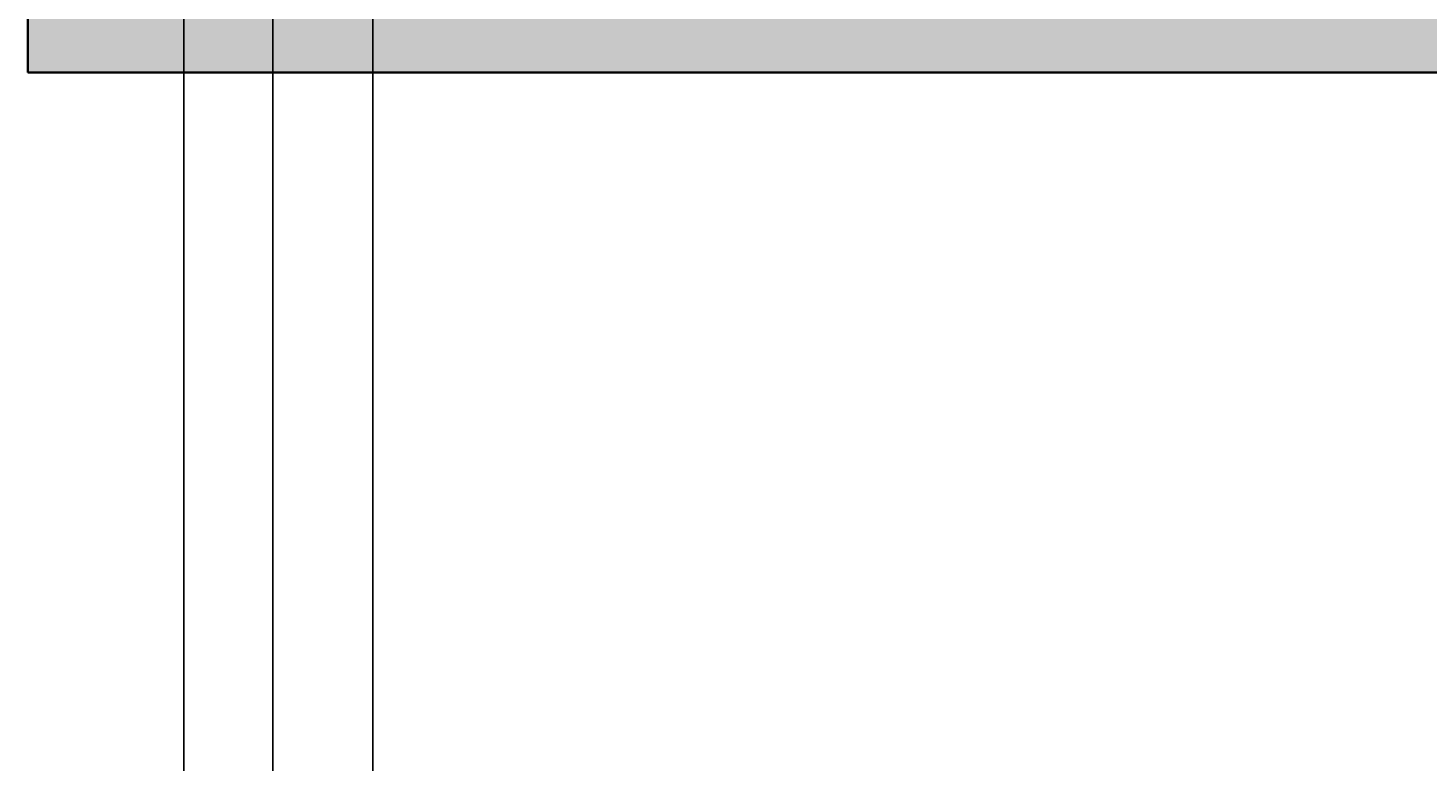
# Model space of a CAD drawing. Units: inches. Extents: x 1567 to 1964, y 1813 to 2447.
# Tile 22 of 28: x 1788 to 1851, y 2228 to 2261. Entities that reach past the tile are written whole.
import ezdxf

# ---------------------------------------------------------------- set-up
doc = ezdxf.new("R2010")
doc.units = ezdxf.units.IN
doc.layers.add('A-ANNO-DIMS', color=2, linetype='Continuous', lineweight=18)
doc.layers.add('A-WALL', color=7, linetype='Continuous', lineweight=35)
doc.layers.add('A-WALL-PATT', color=251, linetype='Continuous', lineweight=13, true_color=0x636466)
doc.styles.get("Standard").update_dxf_attribs({"font": 'arial.ttf'})
doc.dimstyles.get("Standard").update_dxf_attribs({"dimtxt": 0.18, "dimasz": 0.18, "dimexe": 0.18, "dimexo": 0.0625, "dimgap": 0.09, "dimtad": 0, "dimtih": 1, "dimtoh": 1, "dimdec": 4, "dimzin": 0, "dimdsep": 46, "dimtxsty": 'Standard', "dimcen": 0.09, "dimadec": 0, "dimazin": 0, "dimtfac": 1, "dimtdec": 4, "dimtofl": 0, "dimtmove": 0, "dimatfit": 3, "dimfxl": 1, "dimtolj": 1, "dimtzin": 0, "dimarcsym": 0})

# ---------------------------------------------------------------- blocks, each defined once
blk = doc.blocks.new('*D54')
at = {"layer": 'A-ANNO-DIMS', "color": 0, "lineweight": -2, "transparency": 16777216}
for p, q in [((1711.43, 1964.352), (1711.43, 2447.12)), ((1711.61, 2446.94), (1753.211, 2446.94)), ((1795.25, 2446.94), (1753.648, 2446.94)), ((1795.43, 1964.352), (1795.43, 2447.12))]:
    blk.add_line(p, q, dxfattribs=at)
at = {"layer": 'A-ANNO-DIMS', "color": 0, "transparency": 16777216}
for points in [[(1711.61, 2446.97), (1711.61, 2446.91), (1711.43, 2446.94)], [(1795.25, 2446.97), (1795.25, 2446.91), (1795.43, 2446.94)]]:
    blk.add_solid(points, dxfattribs=at)
at = {"layer": 'Defpoints', "color": 0, "transparency": 16777216}
for p in [(1795.43, 2446.94), (1711.43, 1964.29), (1795.43, 1964.29)]:
    blk.add_point(p, dxfattribs=at)
at = {"layer": 'A-ANNO-DIMS', "color": 0, "transparency": 16777216, "insert": (1753.43, 2446.94), "char_height": 0.18, "attachment_point": 5}
blk.add_mtext('\\A1;84', dxfattribs=at)
blk = doc.blocks.new('*D55')
at = {"layer": 'A-ANNO-DIMS', "color": 0, "lineweight": -2, "transparency": 16777216}
for p, q in [((1795.43, 1964.352), (1795.43, 2447.12)), ((1795.61, 2446.94), (1797.277, 2446.94)), ((1799.25, 2446.94), (1797.582, 2446.94)), ((1799.43, 1967.352), (1799.43, 2447.12))]:
    blk.add_line(p, q, dxfattribs=at)
at = {"layer": 'A-ANNO-DIMS', "color": 0, "transparency": 16777216}
for points in [[(1795.61, 2446.97), (1795.61, 2446.91), (1795.43, 2446.94)], [(1799.25, 2446.97), (1799.25, 2446.91), (1799.43, 2446.94)]]:
    blk.add_solid(points, dxfattribs=at)
at = {"layer": 'Defpoints', "color": 0, "transparency": 16777216}
for p in [(1799.43, 2446.94), (1799.43, 1967.29), (1795.43, 1964.29)]:
    blk.add_point(p, dxfattribs=at)
at = {"layer": 'A-ANNO-DIMS', "color": 0, "transparency": 16777216, "insert": (1797.43, 2446.94), "char_height": 0.18, "attachment_point": 5}
blk.add_mtext('\\A1;4', dxfattribs=at)
blk = doc.blocks.new('*D70')
at = {"layer": 'A-ANNO-DIMS', "color": 0, "lineweight": -2, "transparency": 16777216}
for p, q in [((1799.43, 1967.352), (1799.43, 2447.12)), ((1799.61, 2446.94), (1801.421, 2446.94)), ((1803.75, 2446.94), (1801.938, 2446.94)), ((1803.93, 1967.352), (1803.93, 2447.12))]:
    blk.add_line(p, q, dxfattribs=at)
at = {"layer": 'A-ANNO-DIMS', "color": 0, "transparency": 16777216}
for points in [[(1799.61, 2446.97), (1799.61, 2446.91), (1799.43, 2446.94)], [(1803.75, 2446.97), (1803.75, 2446.91), (1803.93, 2446.94)]]:
    blk.add_solid(points, dxfattribs=at)
at = {"layer": 'Defpoints', "color": 0, "transparency": 16777216}
for p in [(1803.93, 2446.94), (1799.43, 1967.29), (1803.93, 1967.29)]:
    blk.add_point(p, dxfattribs=at)
at = {"layer": 'A-ANNO-DIMS', "color": 0, "transparency": 16777216, "insert": (1801.68, 2446.94), "char_height": 0.18, "attachment_point": 5}
blk.add_mtext('\\A1;4.5', dxfattribs=at)
blk = doc.blocks.new('*D71')
at = {"layer": 'A-ANNO-DIMS', "color": 0, "lineweight": -2, "transparency": 16777216}
for p, q in [((1799.43, 1910.752), (1799.43, 2447.12)), ((1799.61, 2446.94), (1861.648, 2446.94)), ((1924.25, 2446.94), (1862.211, 2446.94)), ((1924.43, 1910.752), (1924.43, 2447.12))]:
    blk.add_line(p, q, dxfattribs=at)
at = {"layer": 'A-ANNO-DIMS', "color": 0, "transparency": 16777216}
for points in [[(1799.61, 2446.97), (1799.61, 2446.91), (1799.43, 2446.94)], [(1924.25, 2446.97), (1924.25, 2446.91), (1924.43, 2446.94)]]:
    blk.add_solid(points, dxfattribs=at)
at = {"layer": 'Defpoints', "color": 0, "transparency": 16777216}
for p in [(1924.43, 2446.94), (1799.43, 1910.69), (1924.43, 1910.69)]:
    blk.add_point(p, dxfattribs=at)
at = {"layer": 'A-ANNO-DIMS', "color": 0, "transparency": 16777216, "insert": (1861.93, 2446.94), "char_height": 0.18, "attachment_point": 5}
blk.add_mtext('\\A1;125', dxfattribs=at)

msp = doc.modelspace()

# ---------------------------------------------------------------- hatches: boundary and pattern name
at = {"layer": 'A-WALL-PATT'}
h = msp.add_hatch(color=256, dxfattribs=at)
h.dxf.hatch_style = 1
h.paths.add_polyline_path([(1606.4295, 2407.29), (1654.4295, 2407.29), (1654.4295, 2416.29), (1597.4295, 2416.29), (1597.4295, 2217.29), (1606.4295, 2217.29), (1606.4295, 2259.29), (1738.4295, 2259.29), (1738.4295, 2247.29), (1742.4295, 2247.29), (1742.4295, 2259.29), (1742.4295, 2272.29), (1738.4295, 2272.29), (1738.4295, 2263.29), (1606.4295, 2263.29)])
h.paths.add_polyline_path([(1753.4295, 2416.29), (1690.4295, 2416.29), (1690.4295, 2407.29), (1738.4295, 2407.29), (1738.4295, 2308.29), (1742.4295, 2308.29), (1742.4295, 2331.29), (1746.9295, 2331.29), (1746.9295, 2335.29), (1742.4295, 2335.29), (1742.4295, 2407.29), (1753.4295, 2407.29)])
h.paths.add_polyline_path([(1840.4295, 2416.29), (1777.4295, 2416.29), (1777.4295, 2407.29), (1788.4295, 2407.29), (1788.4295, 2335.29), (1776.9295, 2335.29), (1776.9295, 2331.29), (1788.4295, 2331.29), (1788.4295, 2308.29), (1792.4295, 2308.29), (1792.4295, 2407.29), (1840.4295, 2407.29)])
h.paths.add_polyline_path([(1933.4295, 2416.29), (1876.4295, 2416.29), (1876.4295, 2407.29), (1924.4295, 2407.29), (1924.4295, 2263.29), (1792.4295, 2263.29), (1792.4295, 2272.29), (1788.4295, 2272.29), (1788.4295, 2259.29), (1872.4295, 2259.29), (1872.4295, 2171.29), (1880.9295, 2171.29), (1880.9295, 2175.29), (1876.4295, 2175.29), (1876.4295, 2259.29), (1924.4295, 2259.29), (1924.4295, 2229.29), (1933.4295, 2229.29)])
h.paths.add_polyline_path([(1933.4295, 2205.29), (1924.4295, 2205.29), (1924.4295, 2175.29), (1910.9295, 2175.29), (1910.9295, 2171.29), (1924.4295, 2171.29), (1924.4295, 2127.29), (1844.4295, 2127.29), (1844.4295, 2123.29), (1924.4295, 2123.29), (1924.4295, 2063.29), (1933.4295, 2063.29)])
h.paths.add_polyline_path([(1799.4295, 2123.29), (1808.4295, 2123.29), (1808.4295, 2127.29), (1781.4295, 2127.29), (1781.4295, 2123.29), (1795.4295, 2123.29), (1795.4295, 1964.29), (1711.4295, 1964.29), (1711.4295, 2123.29), (1751.4295, 2123.29), (1751.4295, 2127.29), (1742.4295, 2127.29), (1742.4295, 2139.29), (1738.4295, 2139.29), (1738.4295, 2127.29), (1678.4295, 2127.29), (1678.4295, 2123.29), (1702.4295, 2123.29), (1702.4295, 1913.29), (1678.4295, 1913.29), (1678.4295, 1904.29), (1711.4295, 1904.29), (1711.4295, 1960.29), (1795.4295, 1960.29), (1795.4295, 1906.69), (1929.4295, 1906.69), (1929.4295, 1848.29), (1601.4295, 1848.29), (1601.4295, 1904.29), (1630.4295, 1904.29), (1630.4295, 1913.29), (1606.4295, 1913.29), (1606.4295, 2123.29), (1630.4295, 2123.29), (1630.4295, 2127.29), (1606.4295, 2127.29), (1606.4295, 2169.29), (1597.4295, 2169.29), (1597.4295, 1844.29), (1933.4295, 1844.29), (1933.4295, 2027.29), (1924.4295, 2027.29), (1924.4295, 1967.29), (1833.9295, 1967.29), (1833.9295, 1963.29), (1924.4295, 1963.29), (1924.4295, 1910.69), (1799.4295, 1910.69), (1799.4295, 1963.29), (1803.9295, 1963.29), (1803.9295, 1967.29), (1799.4295, 1967.29)])

# ---------------------------------------------------------------- linework, layer by layer
at = {"layer": 'A-WALL'}
for p, q in [((1788.4295, 2272.29), (1788.4295, 2259.29)), ((1788.4295, 2259.29), (1872.4295, 2259.29))]:
    msp.add_line(p, q, dxfattribs=at)

# ---------------------------------------------------------------- dimensions: what is measured, and where the dimension line sits
at = {"layer": 'A-ANNO-DIMS'}
for base, p1, p2, override, picture, middle in [((1795.4295, 2446.94), (1711.4295, 1964.29), (1795.4295, 1964.29), {"dimdec": 0, "dimlfac": 1, "dimrnd": 0, "dimzin": 0, "dimdsep": 46, "dimlunit": 2}, '*D54', (1753.4295, 2446.94)), ((1799.4295, 2446.94), (1795.4295, 1964.29), (1799.4295, 1967.29), {"dimdec": 0, "dimlfac": 1, "dimrnd": 0, "dimzin": 0, "dimdsep": 46, "dimlunit": 2}, '*D55', (1797.4295, 2446.94)), ((1803.9295, 2446.94), (1799.4295, 1967.29), (1803.9295, 1967.29), {"dimdec": 1, "dimlfac": 1, "dimrnd": 0, "dimzin": 0, "dimdsep": 46, "dimlunit": 2}, '*D70', (1801.6795, 2446.94)), ((1924.4295, 2446.94), (1799.4295, 1910.69), (1924.4295, 1910.69), {"dimdec": 0, "dimlfac": 1, "dimrnd": 0, "dimzin": 0, "dimdsep": 46, "dimlunit": 2}, '*D71', (1861.9295, 2446.94))]:
    dim = msp.add_linear_dim(base=base, p1=p1, p2=p2, dimstyle='Standard', override=override, dxfattribs=at)
    dim.commit()
    dim.dimension.update_dxf_attribs({"geometry": picture, "text_midpoint": middle})

doc.saveas('drawing.dxf')
